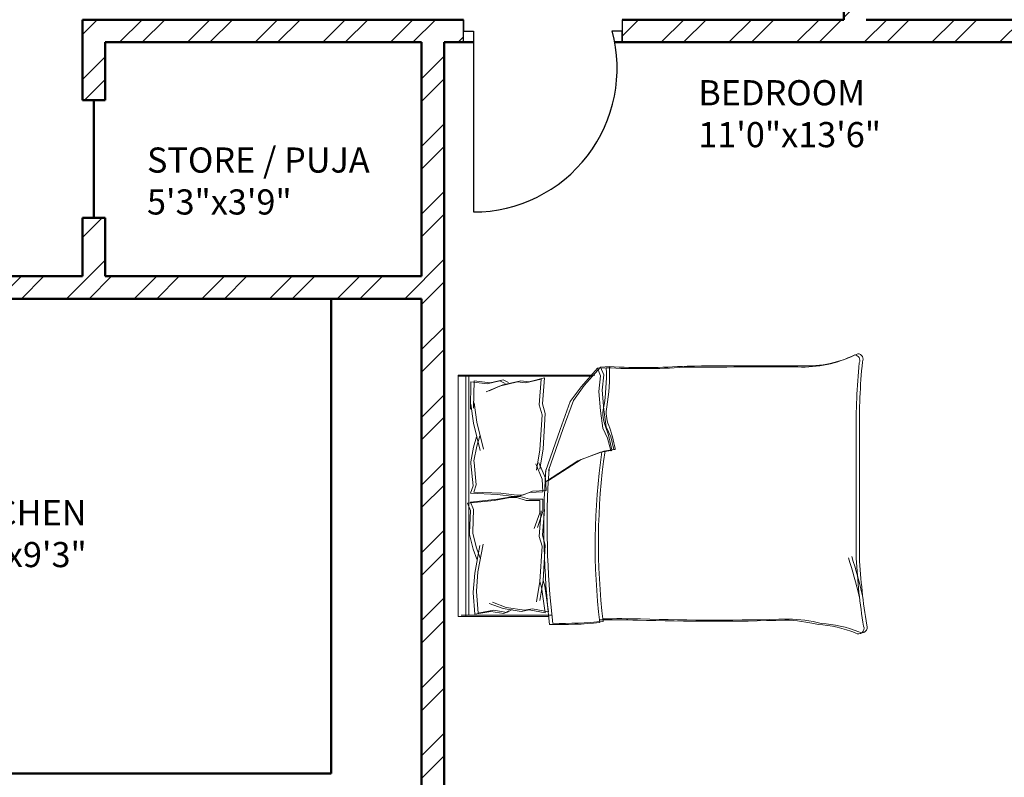
# Model space of a CAD drawing. Units: inches. Extents: x 963 to 2075, y 289 to 2657.
# Tile 46 of 98: x 1689 to 1885, y 1563 to 1714. Entities that reach past the tile are written whole.
import ezdxf

# ---------------------------------------------------------------- set-up
doc = ezdxf.new("R2010")
doc.units = ezdxf.units.IN
for name, color, linetype, lineweight in [('A-AREA-IDEN', 7, 'Continuous', 18), ('A-DOOR', 4, 'Continuous', 25), ('A-FURN', 8, 'Continuous', 18), ('A-WALL', 7, 'Continuous', 50), ('A-WALL-PATT', 8, 'Continuous', 13)]:
    doc.layers.add(name, color=color, linetype=linetype, lineweight=lineweight)
doc.styles.get("Standard").update_dxf_attribs({"font": 'arial.ttf'})

# ---------------------------------------------------------------- blocks, each defined once
blk = doc.blocks.new('BED-DOUBLE')
for p, q in [((1236.12, 2450.52), (1254.23, 2450.52)), ((1236.12, 2450.52), (1254.23, 2450.52)), ((1236.76, 2450.75), (1254.87, 2450.75)), ((1236.76, 2450.75), (1254.87, 2450.75)), ((1237.61, 2444.71), (1236.89, 2449.81)), ((1236.89, 2449.81), (1240.07, 2449.23)), ((1237.61, 2444.71), (1236.89, 2449.81)), ((1236.89, 2449.81), (1240.07, 2449.23)), ((1238.25, 2444.94), (1237.53, 2450.04)), ((1237.53, 2450.04), (1240.71, 2449.46)), ((1238.25, 2444.94), (1237.53, 2450.04)), ((1237.53, 2450.04), (1240.71, 2449.46)), ((1240.71, 2449.46), (1242.3, 2449.75)), ((1240.71, 2449.46), (1242.3, 2449.75)), ((1242.3, 2449.75), (1245.92, 2449.17)), ((1242.3, 2449.75), (1245.92, 2449.17)), ((1245.13, 2449.96), (1244.12, 2449.38)), ((1245.13, 2449.96), (1244.12, 2449.38)), ((1245.77, 2450.18), (1244.76, 2449.61)), ((1245.77, 2450.18), (1244.76, 2449.61)), ((1247.74, 2449.52), (1245.13, 2449.96)), ((1247.74, 2449.52), (1245.13, 2449.96)), ((1248.37, 2449.75), (1245.77, 2450.18)), ((1248.37, 2449.75), (1245.77, 2450.18)), ((1250.92, 2450.1), (1247.74, 2449.52)), ((1250.92, 2450.1), (1247.74, 2449.52)), ((1251.56, 2450.33), (1248.37, 2449.75)), ((1251.56, 2450.33), (1248.37, 2449.75)), ((1250.89, 2450.1), (1251.22, 2445.82)), ((1250.89, 2450.1), (1251.22, 2445.82)), ((1251.53, 2450.32), (1251.86, 2446.04)), ((1251.53, 2450.32), (1251.86, 2446.04)), ((1252.7, 2450.52), (1252.7, 2402.73)), ((1252.7, 2450.52), (1252.7, 2402.73)), ((1253.34, 2450.75), (1253.34, 2402.96)), ((1253.34, 2450.75), (1253.34, 2402.96)), ((1254.87, 2450.75), (1254.87, 2402.73)), ((1239.24, 2447.84), (1238.58, 2443.81)), ((1239.24, 2447.84), (1238.58, 2443.81)), ((1240.07, 2449.23), (1241.66, 2449.52)), ((1240.07, 2449.23), (1241.66, 2449.52)), ((1241.66, 2449.52), (1245.28, 2448.94)), ((1241.66, 2449.52), (1245.28, 2448.94)), ((1245.28, 2448.94), (1248.02, 2447.93)), ((1245.28, 2448.94), (1248.02, 2447.93)), ((1245.92, 2449.17), (1248.66, 2448.16)), ((1245.92, 2449.17), (1248.66, 2448.16)), ((1238.6, 2447.61), (1237.94, 2443.58)), ((1238.6, 2447.61), (1237.94, 2443.58)), ((1251.21, 2445.71), (1250.92, 2441.89)), ((1251.21, 2445.71), (1250.92, 2441.89)), ((1251.22, 2445.82), (1251.21, 2445.71)), ((1251.22, 2445.82), (1251.21, 2445.71)), ((1251.84, 2445.94), (1251.56, 2442.11)), ((1251.84, 2445.94), (1251.56, 2442.11)), ((1251.86, 2446.04), (1251.84, 2445.94)), ((1251.86, 2446.04), (1251.84, 2445.94)), ((1237.94, 2443.58), (1237.61, 2444.71)), ((1237.94, 2443.58), (1237.61, 2444.71)), ((1238.58, 2443.81), (1238.15, 2436.8)), ((1238.58, 2443.81), (1238.15, 2436.8)), ((1238.58, 2443.81), (1238.25, 2444.94)), ((1238.58, 2443.81), (1238.25, 2444.94)), ((1237.94, 2443.58), (1237.51, 2436.57)), ((1237.94, 2443.58), (1237.51, 2436.57)), ((1250.92, 2441.89), (1249.9, 2436.39)), ((1250.92, 2441.89), (1249.9, 2436.39)), ((1251.56, 2442.11), (1250.54, 2436.62)), ((1251.56, 2442.11), (1250.54, 2436.62)), ((1174.99, 2438.93), (1174.99, 2414.32)), ((1174.99, 2438.93), (1174.99, 2414.32)), ((1175.63, 2439.16), (1175.63, 2414.55)), ((1175.63, 2439.16), (1175.63, 2414.55)), ((1250.48, 2439.14), (1251.21, 2437.12)), ((1250.48, 2439.14), (1251.21, 2437.12)), ((1251.12, 2439.37), (1251.84, 2437.34)), ((1251.12, 2439.37), (1251.84, 2437.34)), ((1237.51, 2436.57), (1238.06, 2434.61)), ((1237.51, 2436.57), (1238.06, 2434.61)), ((1238.15, 2436.8), (1238.7, 2434.84)), ((1238.15, 2436.8), (1238.7, 2434.84)), ((1251.21, 2437.12), (1251.93, 2434.22)), ((1251.21, 2437.12), (1251.93, 2434.23)), ((1251.84, 2437.34), (1252.57, 2434.45)), ((1251.84, 2437.34), (1252.57, 2434.45)), ((1238.06, 2434.61), (1237.66, 2429.48)), ((1238.06, 2434.61), (1237.66, 2429.48)), ((1238.7, 2434.84), (1238.3, 2429.71)), ((1238.7, 2434.84), (1238.3, 2429.71)), ((1251.93, 2434.23), (1251.93, 2433.9)), ((1251.93, 2434.22), (1251.93, 2433.9)), ((1252.57, 2434.13), (1252.42, 2429.69)), ((1252.57, 2434.13), (1252.42, 2429.69)), ((1252.57, 2434.45), (1252.57, 2434.13)), ((1252.57, 2434.45), (1252.57, 2434.13)), ((1237.97, 2429.89), (1239.06, 2433.04)), ((1237.97, 2429.89), (1239.06, 2433.04)), ((1238.61, 2430.12), (1239.7, 2433.26)), ((1238.61, 2430.12), (1239.7, 2433.26)), ((1251.93, 2433.9), (1251.78, 2429.46)), ((1251.93, 2433.9), (1251.78, 2429.46)), ((1238.61, 2427.66), (1238.61, 2430.12)), ((1238.61, 2427.66), (1238.61, 2430.12)), ((1237.97, 2427.43), (1237.97, 2429.89)), ((1237.97, 2427.43), (1237.97, 2429.89)), ((1253, 2428.24), (1247.65, 2427.66)), ((1253, 2428.24), (1247.65, 2427.66)), ((1251.78, 2429.46), (1252.36, 2428.01)), ((1251.78, 2429.46), (1252.36, 2428.01)), ((1252.42, 2429.69), (1253, 2428.24)), ((1252.42, 2429.69), (1253, 2428.24)), ((1240.65, 2427.43), (1237.97, 2427.43)), ((1240.65, 2427.43), (1237.97, 2427.43)), ((1241.29, 2427.66), (1238.61, 2427.66)), ((1241.29, 2427.66), (1238.61, 2427.66)), ((1241.86, 2426.56), (1240.02, 2425.86)), ((1241.86, 2426.56), (1240.02, 2425.86)), ((1242.53, 2426.86), (1240.65, 2427.43)), ((1242.53, 2426.86), (1240.65, 2427.43)), ((1242.49, 2426.79), (1240.66, 2426.09)), ((1242.49, 2426.79), (1240.66, 2426.09)), ((1243.17, 2427.08), (1241.29, 2427.66)), ((1243.17, 2427.08), (1241.29, 2427.66)), ((1243.15, 2426.64), (1241.86, 2426.56)), ((1243.15, 2426.64), (1241.86, 2426.56)), ((1243.79, 2426.87), (1242.49, 2426.79)), ((1243.79, 2426.87), (1242.49, 2426.79)), ((1243.83, 2426.86), (1242.53, 2426.86)), ((1243.83, 2426.86), (1242.53, 2426.86)), ((1246.37, 2426.26), (1243.15, 2426.64)), ((1246.37, 2426.26), (1243.15, 2426.64)), ((1244.47, 2427.08), (1243.17, 2427.08)), ((1244.47, 2427.08), (1243.17, 2427.08)), ((1247, 2426.49), (1243.79, 2426.87)), ((1247, 2426.49), (1243.79, 2426.87)), ((1247.01, 2427.43), (1243.83, 2426.86)), ((1247.01, 2427.43), (1243.83, 2426.86)), ((1247.65, 2427.66), (1244.47, 2427.08)), ((1247.65, 2427.66), (1244.47, 2427.08)), ((1251.74, 2426.02), (1246.37, 2426.26)), ((1251.74, 2426.02), (1246.37, 2426.26)), ((1252.38, 2426.25), (1247, 2426.49)), ((1252.38, 2426.25), (1247, 2426.49)), ((1252.36, 2428.01), (1247.01, 2427.43)), ((1252.36, 2428.01), (1247.01, 2427.43)), ((1251.89, 2424.77), (1252.38, 2426.25)), ((1251.89, 2424.77), (1252.38, 2426.25)), ((1240.02, 2425.86), (1237.34, 2425.7)), ((1240.02, 2425.86), (1237.34, 2425.7)), ((1237.34, 2425.7), (1237.49, 2423.24)), ((1237.34, 2425.7), (1237.49, 2423.24)), ((1240.66, 2426.09), (1237.98, 2425.93)), ((1240.66, 2426.09), (1237.98, 2425.93)), ((1237.98, 2425.93), (1238.13, 2423.47)), ((1237.98, 2425.93), (1238.13, 2423.47)), ((1251.25, 2424.54), (1251.74, 2426.02)), ((1251.25, 2424.54), (1251.74, 2426.02)), ((1251.68, 2420.11), (1251.25, 2424.54)), ((1251.68, 2420.11), (1251.25, 2424.54)), ((1252.31, 2420.34), (1251.89, 2424.77)), ((1252.31, 2420.34), (1251.89, 2424.77)), ((1236.85, 2423.74), (1230.36, 2419.55)), ((1236.85, 2423.74), (1230.36, 2419.55)), ((1237.49, 2423.96), (1231, 2419.77)), ((1237.49, 2423.96), (1231, 2419.77)), ((1237.49, 2423.24), (1238.78, 2420.17)), ((1237.49, 2423.24), (1238.78, 2420.17)), ((1238.13, 2423.47), (1239.42, 2420.4)), ((1238.13, 2423.47), (1239.42, 2420.4)), ((1233.92, 2413.35), (1236.85, 2421.69)), ((1233.92, 2413.35), (1236.85, 2421.69)), ((1234.56, 2413.58), (1237.49, 2421.92)), ((1234.56, 2413.58), (1237.49, 2421.92)), ((1238.6, 2421.43), (1237.94, 2417.4)), ((1238.6, 2421.43), (1237.94, 2417.4)), ((1239.24, 2421.66), (1238.58, 2417.63)), ((1239.24, 2421.66), (1238.58, 2417.63)), ((1252.33, 2420.02), (1252.31, 2420.34)), ((1252.33, 2420.02), (1252.31, 2420.34)), ((1230.36, 2419.55), (1225.87, 2417.84)), ((1230.36, 2419.55), (1225.87, 2417.84)), ((1231, 2419.77), (1226.51, 2418.07)), ((1231, 2419.77), (1226.51, 2418.07)), ((1251.15, 2416.86), (1251.7, 2419.79)), ((1251.15, 2416.86), (1251.7, 2419.79)), ((1251.7, 2419.79), (1251.68, 2420.11)), ((1251.7, 2419.79), (1251.68, 2420.11)), ((1251.79, 2417.09), (1252.33, 2420.02)), ((1251.79, 2417.09), (1252.33, 2420.02)), ((1225.87, 2417.84), (1223.86, 2417.53)), ((1225.87, 2417.84), (1223.86, 2417.53)), ((1223.86, 2417.53), (1224.47, 2415.05)), ((1223.86, 2417.53), (1224.47, 2415.05)), ((1226.51, 2418.07), (1224.49, 2417.76)), ((1226.51, 2418.07), (1224.49, 2417.76)), ((1224.49, 2417.76), (1225.11, 2415.28)), ((1224.49, 2417.76), (1225.11, 2415.28)), ((1237.94, 2417.4), (1237.51, 2410.39)), ((1237.94, 2417.4), (1237.51, 2410.39)), ((1238.58, 2417.63), (1238.15, 2410.62)), ((1238.58, 2417.63), (1238.15, 2410.62)), ((1251.16, 2412.08), (1249.81, 2417.5)), ((1251.16, 2412.08), (1249.81, 2417.5)), ((1251.8, 2412.31), (1250.45, 2417.73)), ((1251.8, 2412.31), (1250.45, 2417.73)), ((1250.56, 2414.79), (1251.15, 2416.86)), ((1250.56, 2414.79), (1251.15, 2416.86)), ((1251.2, 2415.02), (1251.79, 2417.09)), ((1251.2, 2415.02), (1251.79, 2417.09)), ((1224.47, 2415.05), (1225.4, 2413.04)), ((1224.47, 2415.05), (1225.4, 2413.04)), ((1225.11, 2415.28), (1226.04, 2413.27)), ((1225.11, 2415.28), (1226.04, 2413.27)), ((1225.4, 2413.04), (1225.87, 2409.63)), ((1225.4, 2413.04), (1225.87, 2409.63)), ((1226.04, 2413.27), (1226.51, 2409.86)), ((1226.04, 2413.27), (1226.51, 2409.86)), ((1231.9, 2407.77), (1233.92, 2413.35)), ((1231.9, 2407.78), (1233.92, 2413.35)), ((1232.54, 2408), (1234.56, 2413.58)), ((1232.54, 2408), (1234.56, 2413.58)), ((1238.15, 2410.62), (1238.7, 2408.66)), ((1238.15, 2410.62), (1238.7, 2408.66)), ((1251.69, 2408.28), (1251.16, 2412.08)), ((1251.69, 2408.28), (1251.16, 2412.08)), ((1252.33, 2408.51), (1251.8, 2412.31)), ((1252.33, 2408.51), (1251.8, 2412.31)), ((1225.87, 2409.63), (1226.18, 2405.76)), ((1225.87, 2409.63), (1226.18, 2405.76)), ((1226.51, 2409.86), (1226.82, 2405.99)), ((1226.51, 2409.86), (1226.82, 2405.99)), ((1237.51, 2410.39), (1238.06, 2408.43)), ((1237.51, 2410.39), (1238.06, 2408.43)), ((1238.7, 2408.66), (1238.3, 2403.52)), ((1238.7, 2408.66), (1238.3, 2403.52)), ((1251.68, 2403.88), (1251.77, 2409.29)), ((1251.68, 2403.88), (1251.77, 2409.28)), ((1251.77, 2409.29), (1251.69, 2408.28)), ((1251.77, 2409.28), (1251.69, 2408.28)), ((1252.31, 2404.11), (1252.41, 2409.51)), ((1252.31, 2404.11), (1252.41, 2409.51)), ((1252.41, 2409.51), (1252.33, 2408.51)), ((1252.41, 2409.51), (1252.33, 2408.51)), ((1229.74, 2404.83), (1231.9, 2407.78)), ((1229.74, 2404.83), (1231.9, 2407.77)), ((1230.38, 2405.06), (1232.54, 2408)), ((1230.38, 2405.06), (1232.54, 2408)), ((1238.06, 2408.43), (1237.66, 2403.3)), ((1238.06, 2408.43), (1237.66, 2403.3)), ((1226.18, 2405.76), (1225.87, 2402.66)), ((1226.18, 2405.76), (1225.87, 2402.66)), ((1226.49, 2401.13), (1229.74, 2404.83)), ((1226.49, 2401.13), (1229.74, 2404.83)), ((1226.82, 2405.99), (1226.51, 2402.89)), ((1226.82, 2405.99), (1226.51, 2402.89)), ((1227.13, 2401.36), (1230.38, 2405.06)), ((1227.13, 2401.36), (1230.38, 2405.06)), ((1242.4, 2403.88), (1245.98, 2404.69)), ((1242.4, 2403.88), (1245.98, 2404.69)), ((1243.04, 2404.11), (1246.61, 2404.91)), ((1243.04, 2404.11), (1246.61, 2404.91)), ((1245.98, 2404.69), (1248.65, 2405.87)), ((1245.98, 2404.69), (1248.65, 2405.87)), ((1246.61, 2404.91), (1249.29, 2406.1)), ((1246.61, 2404.91), (1249.29, 2406.09)), ((1225.87, 2402.66), (1226.49, 2401.13)), ((1225.87, 2402.66), (1226.49, 2401.13)), ((1226.51, 2402.89), (1227.13, 2401.36)), ((1226.51, 2402.89), (1227.13, 2401.36)), ((1254.23, 2402.73), (1227.62, 2402.73)), ((1254.23, 2402.73), (1227.62, 2402.73)), ((1254.87, 2402.96), (1228.26, 2402.96)), ((1254.87, 2402.96), (1228.26, 2402.96)), ((1237.66, 2403.3), (1240.8, 2404.07)), ((1237.66, 2403.3), (1240.8, 2404.07)), ((1238.3, 2403.52), (1241.44, 2404.3)), ((1238.3, 2403.52), (1241.44, 2404.3)), ((1240.8, 2404.07), (1242.4, 2403.88)), ((1240.8, 2404.07), (1242.4, 2403.88)), ((1241.44, 2404.3), (1243.04, 2404.11)), ((1241.44, 2404.3), (1243.04, 2404.11)), ((1245.89, 2403.67), (1244.85, 2404.18)), ((1245.89, 2403.67), (1244.85, 2404.18)), ((1246.53, 2403.89), (1245.49, 2404.41)), ((1246.53, 2403.89), (1245.49, 2404.41)), ((1248.46, 2404.26), (1245.89, 2403.67)), ((1248.46, 2404.26), (1245.89, 2403.67)), ((1249.1, 2404.49), (1246.53, 2403.89)), ((1249.1, 2404.49), (1246.53, 2403.89)), ((1251.68, 2403.88), (1248.46, 2404.26)), ((1251.68, 2403.88), (1248.46, 2404.26)), ((1252.31, 2404.11), (1249.1, 2404.49)), ((1252.31, 2404.11), (1249.1, 2404.49)), ((1254.87, 2402.73), (1254.23, 2402.73)), ((1224.74, 2401.05), (1226.49, 2401.13, 3.87)), ((1224.74, 2401.05), (1226.49, 2401.13, 3.87)), ((1225.38, 2401.28), (1227.13, 2401.36, 3.87)), ((1225.38, 2401.28), (1227.13, 2401.36, 3.87))]:
    blk.add_line(p, q)
for centre, radius, start, end in [((1174.51, 2452.91), 1.09, 56.1736, 203.4781), ((1174.51, 2452.91), 1.09, 56.1736, 203.4781), ((1175.15, 2453.14), 1.09, 56.1736, 203.4781), ((1175.15, 2453.14), 1.09, 56.1736, 203.4781), ((1183.96, 2475.65), 23.56, 247.9751, 266.652), ((1183.96, 2475.65), 23.56, 247.9751, 266.652), ((1184.6, 2475.88), 23.56, 247.9751, 266.652), ((1184.6, 2475.88), 23.56, 247.9751, 266.652), ((1053.4, 2432.57), 121.76, 2.9958, 9.4091), ((1053.4, 2432.57), 121.76, 2.9958, 9.4091), ((1054.03, 2432.8), 121.76, 2.9958, 9.4091), ((1054.03, 2432.8), 121.76, 2.9958, 9.4091), ((1189.72, 2480.89), 29.63, 256.0648, 268.9113), ((1189.72, 2480.89), 29.63, 256.0648, 268.9113), ((1190.36, 2481.12), 29.63, 256.0648, 268.9113), ((1190.36, 2481.12), 29.63, 256.0648, 268.9113), ((1204.26, 1969.4), 482.31, 88.2277, 91.7185), ((1204.26, 1969.4), 482.31, 88.2277, 91.7185), ((1097.92, 2436.24), 129.02, 351.7845, 6.9006), ((1097.92, 2436.24), 129.02, 351.7845, 6.9006), ((1234.14, 2368.83), 83.31, 88.7218, 95.604), ((1234.14, 2368.83), 83.31, 88.7218, 95.604), ((1098.56, 2436.47), 129.02, 351.7845, 6.9006), ((1098.56, 2436.47), 129.02, 351.7845, 6.9006), ((1234.78, 2369.06), 83.31, 88.7218, 95.604), ((1234.78, 2369.06), 83.31, 88.7218, 95.604), ((1072.18, 2432.64), 164.97, 356.0865, 6.7821), ((1072.18, 2432.64), 164.97, 356.0865, 6.7821), ((1072.82, 2432.86), 164.97, 356.0865, 6.7821), ((1072.82, 2432.86), 164.97, 356.0865, 6.7821), ((1203.62, 1969.17), 482.31, 88.2277, 91.7185), ((1203.62, 1969.17), 482.31, 88.2277, 91.7185), ((1223.06, 2621.3), 170.11, 268.4762, 271.0082), ((1223.06, 2621.3), 170.11, 268.4762, 271.0082), ((1223.7, 2621.53), 170.11, 268.4762, 271.0082), ((1223.7, 2621.53), 170.11, 268.4762, 271.0082), ((1277.94, 2471.22), 106.46, 193.3832, 197.7053), ((1277.94, 2471.22), 106.46, 193.3832, 197.7053), ((1278.58, 2471.44), 106.46, 193.3832, 197.7053), ((1278.58, 2471.44), 106.46, 193.3832, 197.7053), ((1223.79, 2417.36), 0.185, 70.2464, 181.1377), ((1223.79, 2417.36), 0.185, 70.2464, 181.1377), ((1252.75, 2422.84), 29.65, 190.6617, 199.8806), ((1252.75, 2422.84), 29.65, 190.6617, 199.8806), ((1224.43, 2417.59), 0.185, 70.2464, 181.1377), ((1224.43, 2417.59), 0.185, 70.2464, 181.1377), ((1253.39, 2423.07), 29.65, 190.6617, 199.8806), ((1253.39, 2423.07), 29.65, 190.6617, 199.8806), ((1042.6, 2413.07), 133.04, 354.4998, 0.6351), ((1042.6, 2413.07), 133.04, 354.4998, 0.6351), ((1041.96, 2412.84), 133.04, 354.4998, 0.6351), ((1041.96, 2412.84), 133.04, 354.4998, 0.6351), ((1219.17, 2410.25), 6.22, 348.6608, 23.7384), ((1219.17, 2410.25), 6.22, 348.6608, 23.7384), ((1219.81, 2410.48), 6.22, 348.6608, 23.7384), ((1219.81, 2410.48), 6.22, 348.6608, 23.7384), ((1260.89, 2402.67), 36.18, 169.8763, 182.5657), ((1260.89, 2402.67), 36.18, 169.8763, 182.5657), ((1261.53, 2402.9), 36.18, 169.8763, 182.5657), ((1261.53, 2402.9), 36.18, 169.8763, 182.5657), ((1185.57, 2377.84), 23.07, 87.4714, 116.4681), ((1185.57, 2377.84), 23.07, 87.4714, 116.4681), ((1186.21, 2378.07), 23.07, 87.4714, 116.4681), ((1186.21, 2378.07), 23.07, 87.4714, 116.4681), ((1186.41, 6962.74), 4561.86, 270.00217, 270.28689), ((1186.41, 6962.74), 4561.86, 270.00217, 270.28689), ((1187.05, 6962.97), 4561.86, 270.00217, 270.28689), ((1187.05, 6962.97), 4561.86, 270.00217, 270.28689), ((1217.92, 2271.73), 129.5, 86.9791, 93.8365), ((1217.92, 2271.73), 129.5, 86.9791, 93.8365), ((1218.56, 2271.96), 129.5, 86.9791, 93.8365), ((1218.56, 2271.96), 129.5, 86.9791, 93.8365), ((1175.36, 2399.58), 1.1, 152.6588, 266.02), ((1175.36, 2399.58), 1.1, 152.6588, 266.02), ((1176, 2399.81), 1.1, 152.6588, 266.02), ((1176, 2399.81), 1.1, 152.6588, 266.02)]:
    blk.add_arc(centre, radius, start, end)

msp = doc.modelspace()

# ---------------------------------------------------------------- hatches: boundary and pattern name
at = {"layer": 'A-WALL-PATT'}
h = msp.add_hatch(dxfattribs=at)
h.set_pattern_fill('ANSI32', color=256)
h.paths.add_polyline_path([(1296.92, 2558.32), (1203.92, 2558.32), (1203.92, 2493.82), (1191.53, 2493.82), (1191.53, 2489.32), (1211.06, 2489.32), (1211.06, 2492.02), (1211.06, 2493.82), (1208.42, 2493.82), (1208.42, 2553.82), (1292.42, 2553.82), (1292.42, 2538.86), (1296.92, 2538.86)])
h.paths.add_polyline_path([(1442.42, 2558.32), (1349.42, 2558.32), (1349.42, 2538.94), (1353.92, 2538.94), (1353.92, 2553.82), (1437.92, 2553.82), (1437.92, 2493.82), (1434.54, 2493.82), (1434.54, 2489.32), (1448.31, 2489.32), (1448.31, 2491.57), (1448.31, 2493.82), (1442.42, 2493.82)])
h.paths.add_polyline_path([(1415.55, 2491.57), (1415.55, 2493.82), (1340.94, 2493.82), (1340.94, 2489.32), (1371.92, 2489.32), (1371.92, 2378.32), (1367.6, 2378.32), (1367.6, 2373.82), (1371.92, 2373.82), (1371.92, 2355.19), (1376.42, 2355.19), (1376.42, 2489.32), (1415.55, 2489.32)])
h.paths.add_polyline_path([(1304.94, 2491.57), (1304.94, 2493.82), (1296.92, 2493.82), (1296.92, 2514.86), (1292.42, 2514.86), (1292.42, 2493.82), (1232.81, 2493.82), (1232.81, 2489.32), (1256.42, 2489.32), (1256.42, 2327.32), (1253.71, 2327.32), (1253.71, 2322.82), (1328.42, 2322.82), (1328.42, 2331.15), (1323.92, 2331.15), (1323.92, 2327.32), (1260.92, 2327.32), (1260.92, 2373.82), (1323.92, 2373.82), (1323.92, 2357.81), (1328.42, 2357.81), (1328.42, 2373.82), (1346.01, 2373.82), (1346.01, 2376.07), (1346.01, 2378.32), (1260.92, 2378.32), (1260.92, 2489.32), (1304.94, 2489.32)])
h.paths.add_polyline_path([(1226.65, 2327.32), (1124.42, 2327.32), (1124.42, 2347.45), (1119.92, 2347.45), (1119.92, 2322.82), (1163.42, 2322.82), (1163.42, 2305.43), (1165.67, 2305.43), (1167.92, 2305.43), (1167.92, 2322.82), (1226.65, 2322.82), (1226.65, 2325.07)])
h.paths.add_polyline_path([(1095.92, 2489.32), (1124.42, 2489.32), (1131.53, 2489.32), (1131.53, 2491.57), (1131.53, 2493.82), (1119.92, 2493.82), (1091.42, 2493.82), (1091.42, 2417.32), (1095.92, 2417.32), (1119.92, 2417.32), (1119.92, 2407.45), (1124.42, 2407.45), (1124.42, 2421.82), (1095.92, 2421.82)])
h.paths.add_polyline_path([(1512.92, 2558.32), (1508.42, 2558.32), (1508.42, 2493.82), (1503.4, 2493.82), (1503.4, 2489.32), (1508.42, 2489.32), (1508.42, 2327.32), (1376.42, 2327.32), (1376.42, 2330.27), (1371.92, 2330.27), (1371.92, 2298.74), (1376.42, 2298.74), (1376.42, 2322.82), (1508.42, 2322.82), (1508.42, 2165.32), (1504.26, 2165.32), (1504.26, 2160.82), (1508.42, 2160.82), (1508.42, 2108.32), (1512.92, 2108.32), (1512.92, 2160.82), (1516.18, 2160.82), (1516.18, 2163.07), (1516.18, 2165.32), (1512.92, 2165.32), (1512.92, 2322.82), (1644.92, 2322.82), (1644.92, 2298.74), (1649.42, 2298.74), (1649.42, 2322.82), (1649.42, 2330.94), (1647.17, 2330.94), (1644.92, 2330.94), (1644.92, 2327.32), (1512.92, 2327.32), (1512.92, 2489.32), (1516.76, 2489.32), (1516.76, 2491.57), (1516.76, 2493.82), (1512.92, 2493.82)])
h.paths.add_polyline_path([(1671.92, 2558.32), (1578.92, 2558.32), (1578.92, 2493.82), (1573.53, 2493.82), (1573.53, 2489.32), (1586.54, 2489.32), (1586.54, 2491.57), (1586.54, 2493.82), (1583.42, 2493.82), (1583.42, 2553.82), (1667.42, 2553.82), (1667.42, 2541.11), (1671.92, 2541.11)])
h.paths.add_polyline_path([(1681.26, 2493.82), (1671.92, 2493.82), (1671.92, 2517.11), (1667.42, 2517.11), (1667.42, 2493.82), (1610.22, 2493.82), (1610.22, 2489.32), (1644.92, 2489.32), (1644.92, 2357.87), (1649.42, 2357.87), (1649.42, 2373.82), (1652.2, 2373.82), (1652.2, 2375.83), (1652.2, 2378.32), (1649.42, 2378.32), (1649.42, 2489.32), (1681.26, 2489.32), (1681.26, 2491.57)])
h.paths.add_polyline_path([(1821.92, 2558.32), (1728.92, 2558.32), (1728.92, 2541), (1733.42, 2541), (1733.42, 2553.82), (1817.42, 2553.82), (1817.42, 2493.82), (1813.51, 2493.82), (1813.51, 2489.32), (1830.08, 2489.32), (1830.08, 2491.57), (1830.08, 2493.82), (1821.92, 2493.82)])
h.paths.add_polyline_path([(1794.24, 2493.82), (1717.26, 2493.82), (1717.26, 2489.32), (1760.42, 2489.32), (1760.42, 2378.32), (1674.4, 2378.32), (1674.4, 2373.82), (1692.92, 2373.82), (1692.92, 2356.95), (1697.42, 2356.95), (1697.42, 2373.82), (1760.42, 2373.82), (1760.42, 2327.32), (1697.42, 2327.32), (1697.42, 2333.34), (1692.92, 2333.34), (1692.92, 2322.82), (1768.04, 2322.82), (1768.04, 2325.07), (1768.04, 2327.32), (1764.92, 2327.32), (1764.92, 2489.32), (1794.24, 2489.32)])
h.paths.add_polyline_path([(1733.42, 2517), (1728.92, 2517), (1728.92, 2493.82), (1733.42, 2493.82)], flags=17)
h.paths.add_polyline_path([(1929.92, 2493.82), (1890.08, 2493.82), (1890.08, 2489.32), (1896.92, 2489.32), (1925.42, 2489.32), (1925.42, 2421.82), (1896.92, 2421.82), (1896.92, 2408.32), (1901.42, 2408.32), (1901.42, 2417.32), (1925.42, 2417.32), (1929.92, 2417.32)])
h.paths.add_polyline_path([(1901.42, 2348.32), (1896.92, 2348.32), (1896.92, 2327.32), (1800.42, 2327.32), (1800.42, 2322.82), (1853.42, 2322.82), (1853.42, 2309.45), (1857.92, 2309.45), (1857.92, 2322.82), (1901.42, 2322.82)])
h.paths.add_polyline_path([(1857.92, 2249.45), (1853.42, 2249.45), (1853.42, 2214.82), (1686.31, 2214.82), (1686.31, 2210.32), (1853.42, 2210.32), (1853.42, 2202.13), (1857.92, 2202.13), (1857.92, 2210.32)])
h.paths.add_polyline_path([(1857.92, 2142.13), (1853.42, 2142.13), (1853.42, 2115.42), (1841.42, 2115.42), (1841.42, 2088.53), (1841.42, 2046.95), (1845.92, 2046.95), (1845.92, 2110.92), (1905.92, 2110.92), (1905.92, 2092.52), (1910.42, 2092.52), (1910.42, 2115.42), (1857.92, 2115.42)])
h.paths.add_polyline_path([(1532.44, 1482.34), (1573.46, 1482.34), (1573.46, 1501), (1532.44, 1501)], flags=9)
h.paths.add_polyline_path([(1438.66, 1486.3), (1479.68, 1486.3), (1479.68, 1504.96), (1438.66, 1504.96)], flags=9)
h.paths.add_polyline_path([(1411.22, 1365.31), (1659.14, 1365.31), (1659.14, 1402.4), (1411.22, 1402.4)], flags=9)
h.paths.add_polyline_path([(1185.67, 2296.3), (1248.16, 2296.3), (1248.16, 2314.95), (1185.67, 2314.95)], flags=9)
h.paths.add_polyline_path([(1177.31, 2187.35), (1216.15, 2187.35), (1216.15, 2206.01), (1177.31, 2206.01)], flags=9)
h.paths.add_polyline_path([(1295.1, 1602.08), (1328.26, 1602.08), (1328.26, 1620.74), (1295.1, 1620.74)], flags=9)
h.paths.add_polyline_path([(1525.13, 2005.99), (1558.39, 2005.99), (1558.39, 2024.65), (1525.13, 2024.65)], flags=9)
h.paths.add_polyline_path([(1459.61, 1977.13), (1472.19, 1977.13), (1472.19, 1987.43), (1459.61, 1987.43)], flags=9)
h.paths.add_polyline_path([(1467.81, 2053.68), (1480.02, 2053.68), (1480.02, 2063.98), (1467.81, 2063.98)], flags=9)
h.paths.add_polyline_path([(1555.18, 2119.02), (1584.56, 2119.02), (1584.56, 2137.68), (1555.18, 2137.68)], flags=25)
h.paths.add_polyline_path([(1405.39, 2115.29), (1444.48, 2115.29), (1444.48, 2133.95), (1405.39, 2133.95)], flags=25)
h.paths.add_polyline_path([(1698.48, 2004.26), (1727.69, 2004.26), (1727.69, 2022.92), (1698.48, 2022.92)], flags=9)
h.paths.add_polyline_path([(1612.16, 1972.86), (1629.02, 1972.86), (1629.02, 1983.16), (1612.16, 1983.16)], flags=9)
h.paths.add_polyline_path([(1608.29, 2060.04), (1625.15, 2060.04), (1625.15, 2070.34), (1608.29, 2070.34)], flags=9)
h.paths.add_polyline_path([(1527.95, 1684.4), (1566.79, 1684.4), (1566.79, 1703.06), (1527.95, 1703.06)], flags=9)
h.paths.add_polyline_path([(1422.79, 1683.59), (1461.63, 1683.59), (1461.63, 1702.25), (1422.79, 1702.25)], flags=9)
h.paths.add_polyline_path([(1531.26, 1732.46), (1574.01, 1732.46), (1574.01, 1751.12), (1531.26, 1751.12)], flags=9)
h.paths.add_polyline_path([(1402.87, 1732.85), (1439.8, 1732.85), (1439.8, 1751.5), (1402.87, 1751.5)], flags=9)
h.paths.add_polyline_path([(1243.12, 1923.13), (1281.96, 1923.13), (1281.96, 1941.79), (1243.12, 1941.79)], flags=9)
h.paths.add_polyline_path([(1181.75, 1792.27), (1244.24, 1792.27), (1244.24, 1810.93), (1181.75, 1810.93)], flags=9)
h.paths.add_polyline_path([(1265.82, 1670.3), (1316.07, 1670.3), (1316.07, 1688.96), (1265.82, 1688.96)], flags=9)
h.paths.add_polyline_path([(1140.26, 1676.05), (1179.1, 1676.05), (1179.1, 1694.71), (1140.26, 1694.71)], flags=9)
h.paths.add_polyline_path([(1107.49, 1490.89), (1143.37, 1490.89), (1143.37, 1509.55), (1107.49, 1509.55)], flags=9)
h.paths.add_polyline_path([(1217.58, 1483.9), (1246.74, 1483.9), (1246.74, 1502.56), (1217.58, 1502.56)], flags=9)
h.paths.add_polyline_path([(1389.21, 1486.92), (1418.37, 1486.92), (1418.37, 1505.58), (1389.21, 1505.58)], flags=9)
h.paths.add_polyline_path([(1672.21, 1602.08), (1705.37, 1602.08), (1705.37, 1620.74), (1672.21, 1620.74)], flags=9)
h.paths.add_polyline_path([(1752.08, 1522.64), (1781.24, 1522.64), (1781.24, 1541.3), (1752.08, 1541.3)], flags=9)
h.paths.add_polyline_path([(1848.27, 1491.26), (1884.16, 1491.26), (1884.16, 1509.92), (1848.27, 1509.92)], flags=9)
h.paths.add_polyline_path([(1822.47, 1685.62), (1861.31, 1685.62), (1861.31, 1704.28), (1822.47, 1704.28)], flags=9)
h.paths.add_polyline_path([(1713.19, 1672.23), (1763.44, 1672.23), (1763.44, 1690.89), (1713.19, 1690.89)], flags=9)
h.paths.add_polyline_path([(1736.62, 1790.58), (1799.11, 1790.58), (1799.11, 1809.24), (1736.62, 1809.24)], flags=9)
h.paths.add_polyline_path([(1691.49, 1916.36), (1730.33, 1916.36), (1730.33, 1935.01), (1691.49, 1935.01)], flags=9)
h.paths.add_polyline_path([(1764.87, 1973.92), (1794.31, 1973.92), (1794.31, 1992.58), (1764.87, 1992.58)], flags=9)
h.paths.add_polyline_path([(1767.85, 2034.02), (1797.29, 2034.02), (1797.29, 2052.67), (1767.85, 2052.67)], flags=9)
h.paths.add_polyline_path([(1851.59, 2060.33), (1880.75, 2060.33), (1880.75, 2078.99), (1851.59, 2078.99)], flags=25)
h.paths.add_polyline_path([(1688.49, 2086.87), (1727.33, 2086.87), (1727.33, 2105.53), (1688.49, 2105.53)], flags=9)
h.paths.add_polyline_path([(1537.74, 2293.58), (1580.49, 2293.58), (1580.49, 2312.24), (1537.74, 2312.24)], flags=25)
h.paths.add_polyline_path([(1425.59, 2296.11), (1468.34, 2296.11), (1468.34, 2314.77), (1425.59, 2314.77)], flags=25)
h.paths.add_polyline_path([(1278.52, 2004.18), (1307.72, 2004.18), (1307.72, 2022.84), (1278.52, 2022.84)], flags=9)
h.paths.add_polyline_path([(1193.28, 1973.63), (1222.72, 1973.63), (1222.72, 1992.29), (1193.28, 1992.29)], flags=9)
h.paths.add_polyline_path([(1192.41, 2040.58), (1221.84, 2040.58), (1221.84, 2059.23), (1192.41, 2059.23)], flags=9)
h.paths.add_polyline_path([(1130.6, 1951.39), (1159.76, 1951.39), (1159.76, 1970.05), (1130.6, 1970.05)], flags=9)
h.paths.add_polyline_path([(1132.83, 2052.49), (1161.98, 2052.49), (1161.98, 2071.15), (1132.83, 2071.15)], flags=9)
h.paths.add_polyline_path([(1265.13, 2334.62), (1315.38, 2334.62), (1315.38, 2353.28), (1265.13, 2353.28)], flags=25)
h.paths.add_polyline_path([(1136.74, 2330.79), (1175.58, 2330.79), (1175.58, 2349.44), (1136.74, 2349.44)], flags=9)
h.paths.add_polyline_path([(1287.42, 2417.2), (1320.58, 2417.2), (1320.58, 2435.86), (1287.42, 2435.86)], flags=25)
h.paths.add_polyline_path([(1430.99, 2329.16), (1469.83, 2329.16), (1469.83, 2347.82), (1430.99, 2347.82)], flags=25)
h.paths.add_polyline_path([(1525.42, 2329.21), (1564.26, 2329.21), (1564.26, 2347.87), (1525.42, 2347.87)], flags=25)
h.paths.add_polyline_path([(1684.52, 2382.8), (1717.68, 2382.8), (1717.68, 2401.46), (1684.52, 2401.46)], flags=25)
h.paths.add_polyline_path([(1704.81, 2340.29), (1755.05, 2340.29), (1755.05, 2358.95), (1704.81, 2358.95)], flags=25)
h.paths.add_polyline_path([(1694.11, 2287.76), (1756.6, 2287.76), (1756.6, 2306.41), (1694.11, 2306.41)], flags=9)
h.paths.add_polyline_path([(1815.78, 2329.86), (1854.62, 2329.86), (1854.62, 2348.52), (1815.78, 2348.52)], flags=9)
h.paths.add_polyline_path([(1842.87, 2514.26), (1878.76, 2514.26), (1878.76, 2532.91), (1842.87, 2532.91)], flags=9)
h.paths.add_polyline_path([(1769.51, 2531.45), (1798.67, 2531.45), (1798.67, 2550.1), (1769.51, 2550.1)], flags=25)
h.paths.add_polyline_path([(1594.77, 2518.47), (1623.93, 2518.47), (1623.93, 2537.13), (1594.77, 2537.13)], flags=25)
h.paths.add_polyline_path([(1520.72, 2516.18), (1556.61, 2516.18), (1556.61, 2534.84), (1520.72, 2534.84)], flags=25)
h.paths.add_polyline_path([(1464.46, 2516.69), (1500.34, 2516.69), (1500.34, 2535.35), (1464.46, 2535.35)], flags=25)
h.paths.add_polyline_path([(1365.7, 2528.97), (1394.85, 2528.97), (1394.85, 2547.63), (1365.7, 2547.63)], flags=25)
h.paths.add_polyline_path([(1222.84, 2516.23), (1252, 2516.23), (1252, 2534.89), (1222.84, 2534.89)], flags=25)
h.paths.add_polyline_path([(1104.55, 2509.6), (1140.43, 2509.6), (1140.43, 2528.26), (1104.55, 2528.26)], flags=9)
h = msp.add_hatch(dxfattribs=at)
h.set_pattern_fill('ANSI32', color=256)
h.paths.add_polyline_path([(1335.97, 2212.57), (1335.97, 2214.82), (1167.92, 2214.82), (1167.92, 2245.43), (1163.42, 2245.43), (1163.42, 2210.32), (1163.42, 2194.81), (1167.92, 2194.81), (1167.92, 2210.32), (1335.97, 2210.32)])
h.paths.add_polyline_path([(1532.44, 1482.34), (1573.46, 1482.34), (1573.46, 1501), (1532.44, 1501)], flags=9)
h.paths.add_polyline_path([(1438.66, 1486.3), (1479.68, 1486.3), (1479.68, 1504.96), (1438.66, 1504.96)], flags=9)
h.paths.add_polyline_path([(1411.22, 1365.31), (1659.14, 1365.31), (1659.14, 1402.4), (1411.22, 1402.4)], flags=9)
h.paths.add_polyline_path([(1185.67, 2296.3), (1248.16, 2296.3), (1248.16, 2314.95), (1185.67, 2314.95)], flags=9)
h.paths.add_polyline_path([(1177.31, 2187.35), (1216.15, 2187.35), (1216.15, 2206.01), (1177.31, 2206.01)], flags=9)
h.paths.add_polyline_path([(1295.1, 1602.08), (1328.26, 1602.08), (1328.26, 1620.74), (1295.1, 1620.74)], flags=9)
h.paths.add_polyline_path([(1525.13, 2005.99), (1558.39, 2005.99), (1558.39, 2024.65), (1525.13, 2024.65)], flags=9)
h.paths.add_polyline_path([(1459.61, 1977.13), (1472.19, 1977.13), (1472.19, 1987.43), (1459.61, 1987.43)], flags=9)
h.paths.add_polyline_path([(1467.81, 2053.68), (1480.02, 2053.68), (1480.02, 2063.98), (1467.81, 2063.98)], flags=9)
h.paths.add_polyline_path([(1555.18, 2119.02), (1584.56, 2119.02), (1584.56, 2137.68), (1555.18, 2137.68)], flags=9)
h.paths.add_polyline_path([(1405.39, 2115.29), (1444.48, 2115.29), (1444.48, 2133.95), (1405.39, 2133.95)], flags=9)
h.paths.add_polyline_path([(1698.48, 2004.26), (1727.69, 2004.26), (1727.69, 2022.92), (1698.48, 2022.92)], flags=9)
h.paths.add_polyline_path([(1612.16, 1972.86), (1629.02, 1972.86), (1629.02, 1983.16), (1612.16, 1983.16)], flags=9)
h.paths.add_polyline_path([(1608.29, 2060.04), (1625.15, 2060.04), (1625.15, 2070.34), (1608.29, 2070.34)], flags=9)
h.paths.add_polyline_path([(1527.95, 1684.4), (1566.79, 1684.4), (1566.79, 1703.06), (1527.95, 1703.06)], flags=9)
h.paths.add_polyline_path([(1422.79, 1683.59), (1461.63, 1683.59), (1461.63, 1702.25), (1422.79, 1702.25)], flags=9)
h.paths.add_polyline_path([(1531.26, 1732.46), (1574.01, 1732.46), (1574.01, 1751.12), (1531.26, 1751.12)], flags=9)
h.paths.add_polyline_path([(1402.87, 1732.85), (1439.8, 1732.85), (1439.8, 1751.5), (1402.87, 1751.5)], flags=9)
h.paths.add_polyline_path([(1243.12, 1923.13), (1281.96, 1923.13), (1281.96, 1941.79), (1243.12, 1941.79)], flags=9)
h.paths.add_polyline_path([(1181.75, 1792.27), (1244.24, 1792.27), (1244.24, 1810.93), (1181.75, 1810.93)], flags=9)
h.paths.add_polyline_path([(1265.82, 1670.3), (1316.07, 1670.3), (1316.07, 1688.96), (1265.82, 1688.96)], flags=9)
h.paths.add_polyline_path([(1140.26, 1676.05), (1179.1, 1676.05), (1179.1, 1694.71), (1140.26, 1694.71)], flags=9)
h.paths.add_polyline_path([(1107.49, 1490.89), (1143.37, 1490.89), (1143.37, 1509.55), (1107.49, 1509.55)], flags=9)
h.paths.add_polyline_path([(1217.58, 1483.9), (1246.74, 1483.9), (1246.74, 1502.56), (1217.58, 1502.56)], flags=9)
h.paths.add_polyline_path([(1389.21, 1486.92), (1418.37, 1486.92), (1418.37, 1505.58), (1389.21, 1505.58)], flags=9)
h.paths.add_polyline_path([(1672.21, 1602.08), (1705.37, 1602.08), (1705.37, 1620.74), (1672.21, 1620.74)], flags=9)
h.paths.add_polyline_path([(1752.08, 1522.64), (1781.24, 1522.64), (1781.24, 1541.3), (1752.08, 1541.3)], flags=9)
h.paths.add_polyline_path([(1848.27, 1491.26), (1884.16, 1491.26), (1884.16, 1509.92), (1848.27, 1509.92)], flags=9)
h.paths.add_polyline_path([(1822.47, 1685.62), (1861.31, 1685.62), (1861.31, 1704.28), (1822.47, 1704.28)], flags=9)
h.paths.add_polyline_path([(1713.19, 1672.23), (1763.44, 1672.23), (1763.44, 1690.89), (1713.19, 1690.89)], flags=9)
h.paths.add_polyline_path([(1736.62, 1790.58), (1799.11, 1790.58), (1799.11, 1809.24), (1736.62, 1809.24)], flags=9)
h.paths.add_polyline_path([(1691.49, 1916.36), (1730.33, 1916.36), (1730.33, 1935.01), (1691.49, 1935.01)], flags=9)
h.paths.add_polyline_path([(1764.87, 1973.92), (1794.31, 1973.92), (1794.31, 1992.58), (1764.87, 1992.58)], flags=9)
h.paths.add_polyline_path([(1767.85, 2034.02), (1797.29, 2034.02), (1797.29, 2052.67), (1767.85, 2052.67)], flags=9)
h.paths.add_polyline_path([(1851.59, 2060.33), (1880.75, 2060.33), (1880.75, 2078.99), (1851.59, 2078.99)], flags=9)
h.paths.add_polyline_path([(1688.49, 2086.87), (1727.33, 2086.87), (1727.33, 2105.53), (1688.49, 2105.53)], flags=9)
h.paths.add_polyline_path([(1537.74, 2293.58), (1580.49, 2293.58), (1580.49, 2312.24), (1537.74, 2312.24)], flags=9)
h.paths.add_polyline_path([(1425.59, 2296.11), (1468.34, 2296.11), (1468.34, 2314.77), (1425.59, 2314.77)], flags=9)
h.paths.add_polyline_path([(1278.52, 2004.18), (1307.72, 2004.18), (1307.72, 2022.84), (1278.52, 2022.84)], flags=9)
h.paths.add_polyline_path([(1193.28, 1973.63), (1222.72, 1973.63), (1222.72, 1992.29), (1193.28, 1992.29)], flags=9)
h.paths.add_polyline_path([(1192.41, 2040.58), (1221.84, 2040.58), (1221.84, 2059.23), (1192.41, 2059.23)], flags=9)
h.paths.add_polyline_path([(1130.6, 1951.39), (1159.76, 1951.39), (1159.76, 1970.05), (1130.6, 1970.05)], flags=9)
h.paths.add_polyline_path([(1132.83, 2052.49), (1161.98, 2052.49), (1161.98, 2071.15), (1132.83, 2071.15)], flags=9)
h.paths.add_polyline_path([(1265.13, 2334.62), (1315.38, 2334.62), (1315.38, 2353.28), (1265.13, 2353.28)], flags=9)
h.paths.add_polyline_path([(1136.74, 2330.79), (1175.58, 2330.79), (1175.58, 2349.44), (1136.74, 2349.44)], flags=9)
h.paths.add_polyline_path([(1287.42, 2417.2), (1320.58, 2417.2), (1320.58, 2435.86), (1287.42, 2435.86)], flags=9)
h.paths.add_polyline_path([(1430.99, 2329.16), (1469.83, 2329.16), (1469.83, 2347.82), (1430.99, 2347.82)], flags=9)
h.paths.add_polyline_path([(1525.42, 2329.21), (1564.26, 2329.21), (1564.26, 2347.87), (1525.42, 2347.87)], flags=9)
h.paths.add_polyline_path([(1684.52, 2382.8), (1717.68, 2382.8), (1717.68, 2401.46), (1684.52, 2401.46)], flags=9)
h.paths.add_polyline_path([(1704.81, 2340.29), (1755.05, 2340.29), (1755.05, 2358.95), (1704.81, 2358.95)], flags=9)
h.paths.add_polyline_path([(1694.11, 2287.76), (1756.6, 2287.76), (1756.6, 2306.41), (1694.11, 2306.41)], flags=9)
h.paths.add_polyline_path([(1815.78, 2329.86), (1854.62, 2329.86), (1854.62, 2348.52), (1815.78, 2348.52)], flags=9)
h.paths.add_polyline_path([(1842.87, 2514.26), (1878.76, 2514.26), (1878.76, 2532.91), (1842.87, 2532.91)], flags=9)
h.paths.add_polyline_path([(1769.51, 2531.45), (1798.67, 2531.45), (1798.67, 2550.1), (1769.51, 2550.1)], flags=9)
h.paths.add_polyline_path([(1594.77, 2518.47), (1623.93, 2518.47), (1623.93, 2537.13), (1594.77, 2537.13)], flags=9)
h.paths.add_polyline_path([(1520.72, 2516.18), (1556.61, 2516.18), (1556.61, 2534.84), (1520.72, 2534.84)], flags=9)
h.paths.add_polyline_path([(1464.46, 2516.69), (1500.34, 2516.69), (1500.34, 2535.35), (1464.46, 2535.35)], flags=9)
h.paths.add_polyline_path([(1365.7, 2528.97), (1394.85, 2528.97), (1394.85, 2547.63), (1365.7, 2547.63)], flags=9)
h.paths.add_polyline_path([(1222.84, 2516.23), (1252, 2516.23), (1252, 2534.89), (1222.84, 2534.89)], flags=9)
h.paths.add_polyline_path([(1104.55, 2509.6), (1140.43, 2509.6), (1140.43, 2528.26), (1104.55, 2528.26)], flags=9)
h = msp.add_hatch(dxfattribs=at)
h.set_pattern_fill('ANSI32', color=256)
h.paths.add_polyline_path([(1910.42, 1929.42), (1910.42, 1963.51), (1905.92, 1963.51), (1905.92, 1929.42), (1845.92, 1929.42), (1845.92, 1993.37), (1843.67, 1993.37), (1841.42, 1993.37), (1841.42, 1951.16), (1841.42, 1924.92), (1853.42, 1924.92), (1853.42, 1913.07), (1857.92, 1913.07), (1857.92, 1924.92), (1910.42, 1924.92)])
h.paths.add_polyline_path([(1857.92, 1853.07), (1853.42, 1853.07), (1853.42, 1826.32), (1841.42, 1826.32), (1674.48, 1826.32), (1674.48, 1821.82), (1853.42, 1821.82), (1857.92, 1821.82)])
h.paths.add_polyline_path([(1857.92, 1821.82), (1853.42, 1821.82), (1853.42, 1807.79), (1857.92, 1807.79)])
h.paths.add_polyline_path([(1857.92, 1747.79), (1853.42, 1747.79), (1853.42, 1713.82), (1809.34, 1713.82), (1809.34, 1709.32), (1905.92, 1709.32), (1905.92, 1688.32), (1910.42, 1688.32), (1910.42, 1713.82), (1857.92, 1713.82)])
h.paths.add_polyline_path([(1830.92, 1542.82), (1837.43, 1542.82), (1837.43, 1545.07), (1837.43, 1547.32), (1823.42, 1547.32), (1823.42, 1545.07), (1823.42, 1542.82), (1826.42, 1542.82), (1826.42, 1482.82), (1742.42, 1482.82), (1742.42, 1505.39), (1737.92, 1505.39), (1737.92, 1478.32), (1830.92, 1478.32)])
h.paths.add_polyline_path([(1938.92, 1619.32), (1934.42, 1619.32), (1910.42, 1619.32), (1910.42, 1628.32), (1908.17, 1628.32), (1905.92, 1628.32), (1905.92, 1614.82), (1934.42, 1614.82), (1934.42, 1547.32), (1905.92, 1547.32), (1899.59, 1547.32), (1899.59, 1542.82), (1910.42, 1542.82), (1938.92, 1542.82)])
h.paths.add_polyline_path([(1803.68, 1547.32), (1773.92, 1547.32), (1773.92, 1709.32), (1777.76, 1709.32), (1777.76, 1713.82), (1701.92, 1713.82), (1701.92, 1697.8), (1706.42, 1697.8), (1706.42, 1709.32), (1769.42, 1709.32), (1769.42, 1662.82), (1706.42, 1662.82), (1706.42, 1674.38), (1701.92, 1674.38), (1701.92, 1662.82), (1675.67, 1662.82), (1675.67, 1658.32), (1769.42, 1658.32), (1769.42, 1547.32), (1729.17, 1547.32), (1729.17, 1542.82), (1737.92, 1542.82), (1737.92, 1529.39), (1742.42, 1529.39), (1742.42, 1542.82), (1803.68, 1542.82)])
h.paths.add_polyline_path([(1595.42, 1542.82), (1599.24, 1542.82), (1599.24, 1547.32), (1584.36, 1547.32), (1584.36, 1542.82), (1590.92, 1542.82), (1590.92, 1436.32), (1595.42, 1436.32), (1595.42, 1440.82)])
h.paths.add_polyline_path([(1693.17, 1547.32), (1649.42, 1547.32), (1649.42, 1658.32), (1652.1, 1658.32), (1652.1, 1660.57), (1652.1, 1662.82), (1649.42, 1662.82), (1649.42, 1680.94), (1647.17, 1680.94), (1644.92, 1680.94), (1644.92, 1547.32), (1622.42, 1547.32), (1622.42, 1545.07), (1622.42, 1542.82), (1649.42, 1542.82), (1679.42, 1542.82), (1679.42, 1529.85), (1681.67, 1529.85), (1683.92, 1529.85), (1683.92, 1542.82), (1693.17, 1542.82), (1693.17, 1545.07)])
h.paths.add_polyline_path([(1683.92, 1505.85), (1679.42, 1505.85), (1679.42, 1483.8), (1595.42, 1483.8), (1595.42, 1479.3), (1683.92, 1479.3)])
h.paths.add_polyline_path([(1402.99, 1547.32), (1376.42, 1547.32), (1376.42, 1675.89), (1374.17, 1675.89), (1371.92, 1675.89), (1371.92, 1662.82), (1368.88, 1662.82), (1368.88, 1658.32), (1371.92, 1658.32), (1371.92, 1547.32), (1335.46, 1547.32), (1335.46, 1542.82), (1337.42, 1542.82), (1337.42, 1526.73), (1341.92, 1526.73), (1341.92, 1542.82), (1371.92, 1542.82), (1402.99, 1542.82)])

# ---------------------------------------------------------------- linework, layer by layer
at = {"layer": 'A-DOOR'}
for p, q in [((1777.76, 1709.32), (1777.76, 1713.82)), ((1777.76, 1713.82), (1777.76, 1711.57)), ((1809.34, 1713.82), (1809.34, 1709.32)), ((1777.76, 1711.57), (1779.76, 1711.57)), ((1779.76, 1711.57), (1779.76, 1675.57)), ((1809.34, 1711.57), (1807.34, 1711.57)), ((1809.34, 1709.32), (1809.34, 1711.57))]:
    msp.add_line(p, q, dxfattribs=at)
msp.add_arc((1779.76, 1704.14), 28.57, 270, 15.0756, dxfattribs=at)
at = {"layer": 'A-WALL'}
for p, q in [((1853.42, 1713.82), (1853.42, 1747.79)), ((1701.92, 1713.82), (1777.76, 1713.82)), ((1701.92, 1713.82), (1701.92, 1697.8)), ((1809.34, 1713.82), (1853.42, 1713.82)), ((1857.92, 1713.82), (1910.42, 1713.82)), ((1769.42, 1709.32), (1706.42, 1709.32)), ((1706.42, 1709.32), (1706.42, 1697.8)), ((1769.42, 1709.32), (1769.42, 1662.82)), ((1773.92, 1709.32), (1773.92, 1547.32)), ((1779.76, 1709.32), (1773.92, 1709.32)), ((1905.92, 1709.32), (1807.85, 1709.32)), ((1706.42, 1697.8), (1701.92, 1697.8)), ((1704.17, 1697.8), (1704.17, 1674.38)), ((1701.92, 1674.38), (1706.42, 1674.38)), ((1701.92, 1674.38), (1701.92, 1662.82)), ((1706.42, 1674.38), (1706.42, 1662.82)), ((1701.92, 1662.82), (1675.67, 1662.82)), ((1769.42, 1662.82), (1706.42, 1662.82)), ((1769.42, 1658.32), (1674, 1658.32)), ((1751.39, 1658.32), (1751.39, 1563.87)), ((1769.42, 1658.32), (1769.42, 1547.32)), ((1751.39, 1563.87), (1649.42, 1563.87))]:
    msp.add_line(p, q, dxfattribs=at)

# ---------------------------------------------------------------- block references
at = {"layer": 'A-FURN', "rotation": 180}
msp.add_blockref('BED-DOUBLE', (3031.54, 4045.86), dxfattribs=at)

# ---------------------------------------------------------------- texts
at = {"layer": 'A-AREA-IDEN', "char_height": 5, "attachment_point": 1}
for s, width, insert in [('BEDROOM\\P11\'0"x13\'6"', 133.3277, (1824.48, 1701.79)), ('STORE / PUJA\\P5\'3"x3\'9"', 92.5143, (1714.76, 1688.4)), ('KITCHEN\\P9\'3"x9\'3"', 120.9099, (1673.97, 1618.25))]:
    msp.add_mtext_dynamic_manual_height_columns(s, width=width, gutter_width=12.5, heights=[0], dxfattribs=dict(at, insert=insert))

doc.saveas('drawing.dxf')
